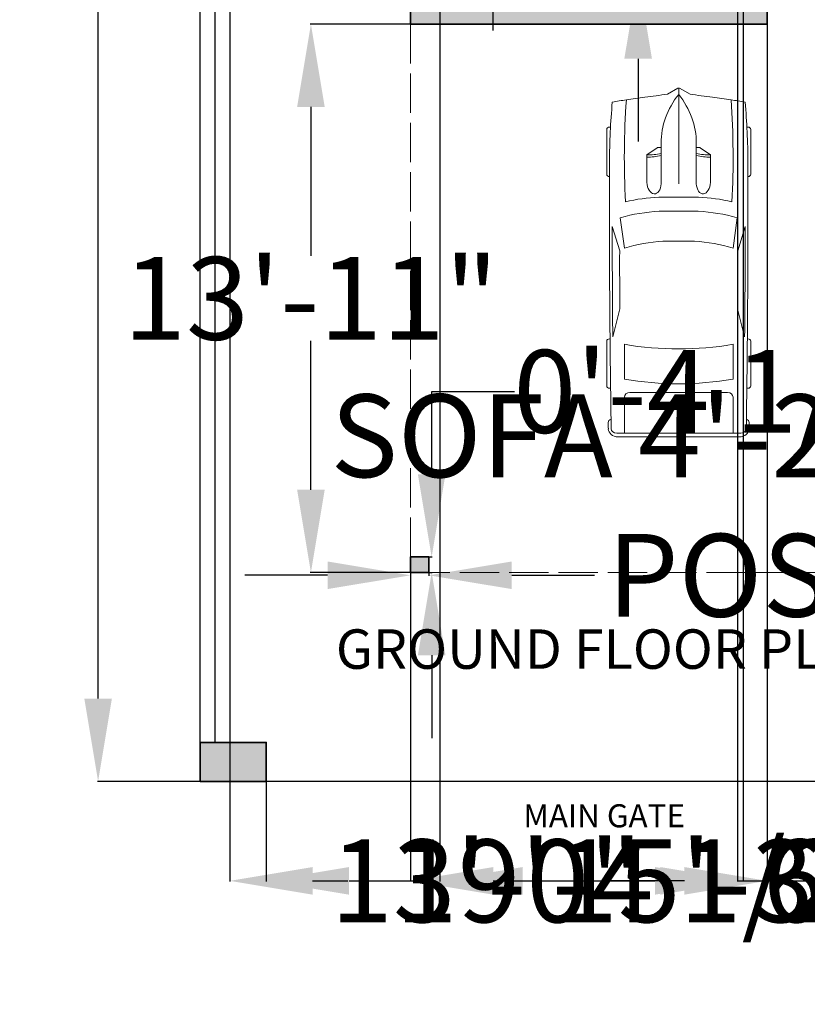
# Model space of a CAD drawing. Units: inches. Extents: x 29 to 6336, y 3 to 2592.
# Tile 1 of 8: x 5292 to 5531, y 1885 to 2184. Entities that reach past the tile are written whole.
import ezdxf

# ---------------------------------------------------------------- set-up
doc = ezdxf.new("R2010")
doc.units = ezdxf.units.IN
doc.header["$MEASUREMENT"] = 0
doc.linetypes.add('ACAD_ISO02W100', pattern=[15, 12, -3])
for name, color, linetype, lineweight in [('A-ANNO-DIMS', 2, 'Continuous', 18), ('A-ANNO-TEXT', 7, 'Continuous', 25), ('A-COLS', 7, 'Continuous', 35), ('A-COLS-PATT', 18, 'Continuous', 13), ('A-EQPM-VEHI', 8, 'Continuous', 18), ('A-FLOR-OVHD', 8, 'ACAD_ISO02W100', 18), ('A-WALL', 7, 'Continuous', 35), ('A-WALL-PATT', 242, 'Continuous', 13), ('C-PROP', 7, 'Continuous', 25)]:
    doc.layers.add(name, color=color, linetype=linetype, lineweight=lineweight)
doc.styles.get("Standard").update_dxf_attribs({"font": 'arial.ttf'})
doc.dimstyles.get("Standard").update_dxf_attribs({"dimtxt": 25.18, "dimasz": 25.18, "dimexe": 0.18, "dimexo": 0.0625, "dimgap": 0.09, "dimtad": 0, "dimtih": 1, "dimtoh": 1, "dimdec": 0, "dimzin": 0, "dimdsep": 46, "dimlunit": 3, "dimtxsty": 'Standard', "dimcen": 0.09, "dimadec": 0, "dimazin": 0, "dimtfac": 1, "dimtdec": 0, "dimtofl": 0, "dimtmove": 0, "dimatfit": 3, "dimfxl": 1, "dimtolj": 1, "dimtzin": 0, "dimarcsym": 0})

# ---------------------------------------------------------------- blocks, each defined once
blk = doc.blocks.new('*D6')
at = {"layer": 'A-ANNO-DIMS', "color": 0, "lineweight": -2, "transparency": 16777216}
for p, q in [((5346.6, 2492.39), (5315.46, 2492.39)), ((5315.64, 2467.21), (5315.64, 2235.26)), ((5315.64, 1977.51), (5315.64, 2209.47)), ((5346.6, 1952.33), (5315.46, 1952.33))]:
    blk.add_line(p, q, dxfattribs=at)
at = {"layer": 'A-ANNO-DIMS', "color": 0, "transparency": 16777216}
for points in [[(5311.44, 2467.21), (5319.83, 2467.21), (5315.64, 2492.39)], [(5311.44, 1977.51), (5319.83, 1977.51), (5315.64, 1952.33)]]:
    blk.add_solid(points, dxfattribs=at)
at = {"layer": 'Defpoints', "color": 0, "transparency": 16777216}
for p in [(5346.66, 2492.39), (5315.64, 1952.33), (5346.66, 1952.33)]:
    blk.add_point(p, dxfattribs=at)
at = {"layer": 'A-ANNO-DIMS', "color": 0, "transparency": 16777216, "insert": (5315.64, 2222.36), "char_height": 25.18, "attachment_point": 5}
blk.add_mtext("\\A1;45'", dxfattribs=at)
blk = doc.blocks.new('*U8')
for p, q in [((21.1, 37.41), (21.1, 36.83)), ((46.55, 38.89), (22.35, 38.89)), ((47.8, 37.39), (47.8, 37.41)), ((135.45, 37.07), (135.45, 37.41)), ((136.7, 38.89), (160.9, 38.89)), ((162.15, 37.41), (162.15, 36.77)), ((87.99, 31.87), (74.76, 35.92)), ((134.31, 35.6), (119.29, 31.78)), ((186.47, -33.5), (186.47, 33.5)), ((188.4, -32.76), (188.4, 32.76)), ((70.03, 31.54), (86.41, 29.35)), ((138.42, 29.35), (157.25, 29.35)), ((186.47, 29.35), (167.01, 29.35)), ((164.52, 26.39), (164.52, -26.39)), ((32.27, 11.63), (36.13, 17.17)), ((36.13, 17.17), (50.94, 17.17)), ((32.12, 9.51), (32.12, 11.15)), ((58.92, -10.77), (58.92, 10.77)), ((3.27, 6.13), (0.1, 0.41)), ((29.77, 9.51), (51.68, 9.51)), ((66.55, -10.53), (66.55, 10.53)), ((82.74, 8.5), (82.74, -8.5)), ((186.47, -10.53), (186.47, 10.53)), ((0, 0), (51.68, 0)), ((0.1, -0.41), (3.27, -6.13)), ((29.77, -9.51), (51.68, -9.51)), ((32.12, -9.51), (32.12, -11.15)), ((32.27, -11.63), (36.13, -17.17)), ((36.13, -17.17), (50.94, -17.17)), ((86.41, -29.35), (70.03, -31.54)), ((87.99, -31.87), (74.76, -35.92)), ((134.31, -35.6), (119.29, -31.78)), ((157.25, -29.35), (138.42, -29.35)), ((167.01, -29.35), (186.47, -29.35)), ((21.1, -37.41), (21.1, -36.83)), ((135.45, -37.07), (135.45, -37.41)), ((162.15, -37.41), (162.15, -36.77)), ((46.55, -38.89), (22.35, -38.89)), ((47.8, -37.39), (47.8, -37.41)), ((136.7, -38.89), (160.9, -38.89))]:
    blk.add_line(p, q)
for centre, major_axis, ratio, start_param, end_param in [((41.19, -490.86), (0, 528.23), 0.842304, 0.00281, 0.075598), ((22.35, 37.41), (0, -1.48), 0.842304, 3.141593, 4.712389), ((64.48, -10555.62), (0, 10593.03), 0.842304, -0.013397, 0.002797), ((46.55, 37.41), (0, 1.48), 0.842304, -1.570796, 0), ((136.7, 37.41), (0, -1.48), 0.842304, 3.141593, 4.712389), ((160.9, 37.41), (0, 1.48), 0.842304, -1.570796, 0), ((180.63, 35.84), (0, 2.22), 0.842304, -0.013017, 1.249894), ((64.48, -10556.36), (0, 10595.31), 0.842304, -0.013397, -0.013017), ((183.98, 32.76), (0, -5.25), 0.842304, 1.570796, 3.128196), ((266.03, -27.52), (0, 313.31), 0.842304, 1.367076, 1.39176), ((64.48, -10555.62), (0, -10591.55), 0.842304, 3.133765, 3.140441), ((183.98, 33.5), (0, -2.96), 0.842304, 1.570796, 3.128196), ((259.18, -27.52), (0, -305.3), 0.842304, 4.528606, 4.561838), ((37.47, -593.96), (0, -623.33), 0.842304, 3.096046, 3.200911), ((134.4, 5.39), (0, -89.78), 0.842304, 4.449482, 4.652344), ((135.29, 5.39), (0, 81.77), 0.842304, 1.245306, 1.50788), ((149.6, 2.8), (0, -79.58), 0.842304, 4.372215, 4.640744), ((95.79, -3666.35), (0, -3698.24), 0.842304, 3.134049, 3.144098), ((17.08, 0), (0, 147.02), 0.842304, 4.511394, 4.913384), ((35.91, 0), (0, 147.02), 0.842304, 4.511394, 4.913384), ((167.01, 26.39), (0, 2.96), 0.842304, 0, 1.570796), ((-204.49, 52.4), (0, -250.96), 0.842304, 1.385369, 1.434372), ((13.04, 17.01), (0, 27.42), 0.842304, 4.435146, 4.718221), ((14.2, 17.01), (0, 27.42), 0.842304, 4.435146, 4.718221), ((50.79, 13.34), (6.34, -0.36), 0.603834, -1.395552, 1.581315), ((32.75, 11.15), (0, 0.74), 0.842304, 0.879714, 1.570796), ((29.77, -46.66), (0, 56.17), 0.842304, 0, 0.590319), ((0.62, 0), (0, -0.74), 0.842304, 4.131459, 5.293319), ((29.77, 46.66), (0, 56.17), 0.842304, 2.551274, 3.141593), ((-204.49, -52.4), (0, 250.96), 0.842304, -1.434372, -1.385369), ((13.04, -17.01), (0, -27.42), 0.842304, 1.564964, 1.848039), ((14.2, -17.01), (0, -27.42), 0.842304, 1.564964, 1.848039), ((135.29, -5.39), (0, -81.77), 0.842304, -1.50788, -1.245306), ((149.6, -2.8), (0, -79.58), 0.842304, -1.499151, -1.230623), ((32.75, -11.15), (0, -0.74), 0.842304, 4.712389, 5.403472), ((134.4, -5.39), (0, -89.78), 0.842304, -1.510751, -1.307889), ((259.18, 27.52), (0, 305.3), 0.842304, 1.721348, 1.754579), ((167.01, -26.39), (0, -2.96), 0.842304, 4.712389, 6.283185), ((266.03, 27.52), (0, 313.31), 0.842304, 1.749832, 1.774517), ((37.47, 593.96), (0, -623.33), 0.842304, -0.059319, 0.045547), ((95.79, 3666.35), (0, -3698.24), 0.842304, -0.002505, 0.007544), ((41.19, 490.86), (0, -528.23), 0.842304, -0.075598, -0.00281), ((64.48, 10555.62), (0, 10593.03), 0.842304, 3.138796, 3.15499), ((64.48, 10555.62), (0, -10591.55), 0.842304, 0.001152, 0.007828), ((180.63, -35.84), (0, -2.22), 0.842304, -1.249894, 0.013017), ((183.98, -33.5), (0, 2.96), 0.842304, 3.15499, 4.712389), ((183.98, -32.76), (0, -5.25), 0.842304, 0.013397, 1.570796), ((22.35, -37.41), (0, 1.48), 0.842304, 1.570796, 3.141593), ((46.55, -37.41), (0, -1.48), 0.842304, 0, 1.570796), ((136.7, -37.41), (0, -1.48), 0.842304, -1.570796, 0), ((160.9, -37.41), (0, 1.48), 0.842304, 3.141593, 4.712389), ((64.48, 10556.36), (0, 10595.31), 0.842304, 3.15461, 3.15499)]:
    blk.add_ellipse(centre, major_axis=major_axis, ratio=ratio, start_param=start_param, end_param=end_param)
at = {"extrusion": (0, 0, -1)}
blk.add_ellipse((50.79, -13.34), major_axis=(6.34, 0.36), ratio=0.603834, start_param=-1.395552, end_param=1.581315, dxfattribs=at)
blk = doc.blocks.new('PORCH-POST')
blk.add_lwpolyline([(5.63, 0), (0, 0), (0, 4.72), (5.63, 4.72)], close=True)
blk = doc.blocks.new('*D25')
at = {"layer": 'A-ANNO-DIMS', "color": 0, "lineweight": -2, "transparency": 16777216}
for p, q in [((5435.68, 2266.92), (5435.68, 2292.1)), ((5435.68, 2292.1), (5460.86, 2292.1)), ((5437.84, 2241.74), (5435.5, 2241.74)), ((5437.84, 2231.12), (5435.5, 2231.12)), ((5435.68, 2205.94), (5435.68, 2180.76))]:
    blk.add_line(p, q, dxfattribs=at)
at = {"layer": 'A-ANNO-DIMS', "color": 0, "transparency": 16777216}
for points in [[(5431.49, 2266.92), (5439.88, 2266.92), (5435.68, 2241.74)], [(5431.49, 2205.94), (5439.88, 2205.94), (5435.68, 2231.12)]]:
    blk.add_solid(points, dxfattribs=at)
at = {"layer": 'Defpoints', "color": 0, "transparency": 16777216}
for p in [(5435.68, 2241.74), (5437.91, 2241.74), (5437.91, 2231.12)]:
    blk.add_point(p, dxfattribs=at)
at = {"layer": 'A-ANNO-DIMS', "color": 0, "transparency": 16777216, "insert": (5576.81, 2292.1), "char_height": 25.18, "attachment_point": 5}
blk.add_mtext('\\A1;0\'-10 1/2" TYP.', dxfattribs=at)
blk = doc.blocks.new('*D28')
at = {"layer": 'A-ANNO-DIMS', "color": 0, "lineweight": -2, "transparency": 16777216}
for p, q in [((5689.81, 2064.89), (5689.81, 2057.28)), ((5739.75, 2064.89), (5739.75, 2057.28)), ((5664.63, 2057.46), (5639.45, 2057.46)), ((5764.93, 2057.46), (5790.11, 2057.46))]:
    blk.add_line(p, q, dxfattribs=at)
at = {"layer": 'A-ANNO-DIMS', "color": 0, "transparency": 16777216}
for points in [[(5664.63, 2061.65), (5664.63, 2053.26), (5689.81, 2057.46)], [(5764.93, 2061.65), (5764.93, 2053.26), (5739.75, 2057.46)]]:
    blk.add_solid(points, dxfattribs=at)
at = {"layer": 'Defpoints', "color": 0, "transparency": 16777216}
for p in [(5689.81, 2064.95), (5739.75, 2064.95), (5689.81, 2057.46)]:
    blk.add_point(p, dxfattribs=at)
at = {"layer": 'A-ANNO-DIMS', "color": 0, "transparency": 16777216, "insert": (5509.91, 2057.46), "char_height": 25.18, "attachment_point": 5}
blk.add_mtext('\\A1;SOFA 4\'-2" TYP.', dxfattribs=at)
blk = doc.blocks.new('*D38')
at = {"layer": 'A-ANNO-DIMS', "color": 0, "lineweight": -2, "transparency": 16777216}
for p, q in [((5410.6, 2015.81), (5410.6, 2014.84)), ((5416.23, 2015.81), (5416.23, 2014.84)), ((5385.42, 2015.02), (5360.24, 2015.02)), ((5441.41, 2015.02), (5466.59, 2015.02))]:
    blk.add_line(p, q, dxfattribs=at)
at = {"layer": 'A-ANNO-DIMS', "color": 0, "transparency": 16777216}
for points in [[(5385.42, 2019.22), (5385.42, 2010.83), (5410.6, 2015.02)], [(5441.41, 2019.22), (5441.41, 2010.83), (5416.23, 2015.02)]]:
    blk.add_solid(points, dxfattribs=at)
at = {"layer": 'Defpoints', "color": 0, "transparency": 16777216}
for p in [(5410.6, 2015.87), (5416.23, 2015.87), (5416.23, 2015.02)]:
    blk.add_point(p, dxfattribs=at)
at = {"layer": 'A-ANNO-DIMS', "color": 0, "transparency": 16777216, "insert": (5624.9, 2015.02), "char_height": 25.18, "attachment_point": 5}
blk.add_mtext('\\A1;POST 0\'-5 1/2" TYP.', dxfattribs=at)
blk = doc.blocks.new('*D39')
at = {"layer": 'A-ANNO-DIMS', "color": 0, "lineweight": -2, "transparency": 16777216}
for p, q in [((5417.07, 2045.77), (5417.07, 2070.95)), ((5417.07, 2070.95), (5442.25, 2070.95)), ((5416.29, 2020.59), (5417.25, 2020.59)), ((5416.29, 2015.87), (5417.25, 2015.87)), ((5417.07, 1990.69), (5417.07, 1965.51))]:
    blk.add_line(p, q, dxfattribs=at)
at = {"layer": 'A-ANNO-DIMS', "color": 0, "transparency": 16777216}
for points in [[(5412.88, 2045.77), (5421.27, 2045.77), (5417.07, 2020.59)], [(5412.88, 1990.69), (5421.27, 1990.69), (5417.07, 2015.87)]]:
    blk.add_solid(points, dxfattribs=at)
at = {"layer": 'Defpoints', "color": 0, "transparency": 16777216}
for p in [(5416.23, 2020.59), (5417.07, 2020.59), (5416.23, 2015.87)]:
    blk.add_point(p, dxfattribs=at)
at = {"layer": 'A-ANNO-DIMS', "color": 0, "transparency": 16777216, "insert": (5548.42, 2070.95), "char_height": 25.18, "attachment_point": 5}
blk.add_mtext('\\A1;0\'-4 1/2" TYP.', dxfattribs=at)
blk = doc.blocks.new('*D42')
at = {"layer": 'A-ANNO-DIMS', "color": 0, "lineweight": -2, "transparency": 16777216}
for p, q in [((5511.77, 2337.07), (5511.77, 1921.9)), ((5355.66, 2328.5), (5355.66, 1921.9)), ((5380.84, 1922.08), (5391.56, 1922.08)), ((5486.59, 1922.08), (5475.87, 1922.08))]:
    blk.add_line(p, q, dxfattribs=at)
at = {"layer": 'A-ANNO-DIMS', "color": 0, "transparency": 16777216}
for points in [[(5380.84, 1926.28), (5380.84, 1917.88), (5355.66, 1922.08)], [(5486.59, 1926.28), (5486.59, 1917.88), (5511.77, 1922.08)]]:
    blk.add_solid(points, dxfattribs=at)
at = {"layer": 'Defpoints', "color": 0, "transparency": 16777216}
for p in [(5511.77, 2337.13), (5355.66, 2328.56), (5511.77, 1922.08)]:
    blk.add_point(p, dxfattribs=at)
at = {"layer": 'A-ANNO-DIMS', "color": 0, "transparency": 16777216, "insert": (5433.71, 1922.08), "char_height": 25.18, "attachment_point": 5}
blk.add_mtext('\\A1;13\'-0"', dxfattribs=at)
blk = doc.blocks.new('*D49')
at = {"layer": 'A-ANNO-DIMS', "color": 0, "lineweight": -2, "transparency": 16777216}
for p, q in [((5419.6, 2191.59), (5419.6, 1921.9)), ((5510.11, 2191.59), (5510.11, 1921.9)), ((5444.78, 1922.08), (5484.93, 1922.08)), ((5510.11, 1922.08), (5535.29, 1922.08))]:
    blk.add_line(p, q, dxfattribs=at)
at = {"layer": 'A-ANNO-DIMS', "color": 0, "transparency": 16777216}
for points in [[(5444.78, 1926.28), (5444.78, 1917.88), (5419.6, 1922.08)], [(5484.93, 1926.28), (5484.93, 1917.88), (5510.11, 1922.08)]]:
    blk.add_solid(points, dxfattribs=at)
at = {"layer": 'Defpoints', "color": 0, "transparency": 16777216}
for p in [(5419.6, 2191.65), (5510.11, 2191.65), (5510.11, 1922.08)]:
    blk.add_point(p, dxfattribs=at)
at = {"layer": 'A-ANNO-DIMS', "color": 0, "transparency": 16777216, "insert": (5598.08, 1922.08), "char_height": 25.18, "attachment_point": 5}
blk.add_mtext('\\A1;7\'-6 1/2"', dxfattribs=at)
blk = doc.blocks.new('*D56')
at = {"layer": 'A-ANNO-DIMS', "color": 0, "lineweight": -2, "transparency": 16777216}
for p, q in [((5366.79, 1952.27), (5366.79, 1921.9)), ((5599.23, 1952.27), (5599.23, 1921.9)), ((5391.97, 1922.08), (5411.52, 1922.08)), ((5574.05, 1922.08), (5554.5, 1922.08))]:
    blk.add_line(p, q, dxfattribs=at)
at = {"layer": 'A-ANNO-DIMS', "color": 0, "transparency": 16777216}
for points in [[(5391.97, 1926.28), (5391.97, 1917.88), (5366.79, 1922.08)], [(5574.05, 1926.28), (5574.05, 1917.88), (5599.23, 1922.08)]]:
    blk.add_solid(points, dxfattribs=at)
at = {"layer": 'Defpoints', "color": 0, "transparency": 16777216}
for p in [(5366.79, 1952.33), (5599.23, 1952.33), (5599.23, 1922.08)]:
    blk.add_point(p, dxfattribs=at)
at = {"layer": 'A-ANNO-DIMS', "color": 0, "transparency": 16777216, "insert": (5483.01, 1922.08), "char_height": 25.18, "attachment_point": 5}
blk.add_mtext('\\A1;19\'-4 1/2"', dxfattribs=at)
blk = doc.blocks.new('*D57')
at = {"layer": 'A-ANNO-DIMS', "color": 0, "lineweight": -2, "transparency": 16777216}
for p, q in [((5410.6, 2015.81), (5410.6, 1921.9)), ((5593.6, 2015.81), (5593.6, 1921.9)), ((5435.78, 1922.08), (5459.94, 1922.08)), ((5568.42, 1922.08), (5544.25, 1922.08))]:
    blk.add_line(p, q, dxfattribs=at)
at = {"layer": 'A-ANNO-DIMS', "color": 0, "transparency": 16777216}
for points in [[(5435.78, 1926.28), (5435.78, 1917.88), (5410.6, 1922.08)], [(5568.42, 1926.28), (5568.42, 1917.88), (5593.6, 1922.08)]]:
    blk.add_solid(points, dxfattribs=at)
at = {"layer": 'Defpoints', "color": 0, "transparency": 16777216}
for p in [(5410.6, 2015.87), (5593.6, 2015.87), (5593.6, 1922.08)]:
    blk.add_point(p, dxfattribs=at)
at = {"layer": 'A-ANNO-DIMS', "color": 0, "transparency": 16777216, "insert": (5502.1, 1922.08), "char_height": 25.18, "attachment_point": 5}
blk.add_mtext('\\A1;15\'-3"', dxfattribs=at)
blk = doc.blocks.new('*D58')
at = {"layer": 'A-ANNO-DIMS', "color": 0, "lineweight": -2, "transparency": 16777216}
for p, q in [((5410.54, 2182.65), (5380.17, 2182.65)), ((5380.35, 2157.47), (5380.35, 2112.21)), ((5380.35, 2041.05), (5380.35, 2086.3)), ((5410.54, 2015.87), (5380.17, 2015.87))]:
    blk.add_line(p, q, dxfattribs=at)
at = {"layer": 'A-ANNO-DIMS', "color": 0, "transparency": 16777216}
for points in [[(5376.16, 2157.47), (5384.55, 2157.47), (5380.35, 2182.65)], [(5376.16, 2041.05), (5384.55, 2041.05), (5380.35, 2015.87)]]:
    blk.add_solid(points, dxfattribs=at)
at = {"layer": 'Defpoints', "color": 0, "transparency": 16777216}
for p in [(5380.35, 2182.65), (5410.6, 2182.65), (5410.6, 2015.87)]:
    blk.add_point(p, dxfattribs=at)
at = {"layer": 'A-ANNO-DIMS', "color": 0, "transparency": 16777216, "insert": (5380.35, 2099.26), "char_height": 25.18, "attachment_point": 5}
blk.add_mtext('\\A1;13\'-11"', dxfattribs=at)
blk = doc.blocks.new('*D59')
at = {"layer": 'A-ANNO-DIMS', "color": 0, "lineweight": -2, "transparency": 16777216}
for p, q in [((5519.11, 2182.59), (5519.11, 1921.9)), ((5592.36, 2182.59), (5592.36, 1921.9)), ((5493.93, 1922.08), (5468.75, 1922.08)), ((5617.54, 1922.08), (5642.72, 1922.08))]:
    blk.add_line(p, q, dxfattribs=at)
at = {"layer": 'A-ANNO-DIMS', "color": 0, "transparency": 16777216}
for points in [[(5493.93, 1926.28), (5493.93, 1917.88), (5519.11, 1922.08)], [(5617.54, 1926.28), (5617.54, 1917.88), (5592.36, 1922.08)]]:
    blk.add_solid(points, dxfattribs=at)
at = {"layer": 'Defpoints', "color": 0, "transparency": 16777216}
for p in [(5519.11, 2182.65), (5592.36, 2182.65), (5592.36, 1922.08)]:
    blk.add_point(p, dxfattribs=at)
at = {"layer": 'A-ANNO-DIMS', "color": 0, "transparency": 16777216, "insert": (5555.73, 1922.08), "char_height": 25.18, "attachment_point": 5}
blk.add_mtext('\\A1;6\'-1"', dxfattribs=at)
blk = doc.blocks.new('*D68')
at = {"layer": 'A-ANNO-DIMS', "color": 0, "lineweight": -2, "transparency": 16777216}
for p, q in [((5479.86, 2259.85), (5479.86, 2285.03)), ((5510.05, 2234.67), (5479.68, 2234.67)), ((5510.05, 2197.33), (5479.68, 2197.33)), ((5479.86, 2172.15), (5479.86, 2146.97))]:
    blk.add_line(p, q, dxfattribs=at)
at = {"layer": 'A-ANNO-DIMS', "color": 0, "transparency": 16777216}
for points in [[(5475.66, 2259.85), (5484.06, 2259.85), (5479.86, 2234.67)], [(5475.66, 2172.15), (5484.06, 2172.15), (5479.86, 2197.33)]]:
    blk.add_solid(points, dxfattribs=at)
at = {"layer": 'Defpoints', "color": 0, "transparency": 16777216}
for p in [(5479.86, 2234.67), (5510.11, 2234.67), (5510.11, 2197.33)]:
    blk.add_point(p, dxfattribs=at)
at = {"layer": 'A-ANNO-DIMS', "color": 0, "transparency": 16777216, "insert": (5479.86, 2216), "char_height": 25.18, "attachment_point": 5}
blk.add_mtext('\\A1;3\'-1 1/2"', dxfattribs=at)

msp = doc.modelspace()

# ---------------------------------------------------------------- hatches: boundary and pattern name
at = {"layer": 'A-COLS-PATT'}
h = msp.add_hatch(color=256, dxfattribs=at)
h.dxf.hatch_style = 1
h.paths.add_polyline_path([(5416.23, 2020.59), (5410.6, 2020.59), (5410.6, 2015.87), (5416.23, 2015.87)])
h.paths.add_polyline_path([(5599.23, 2020.59), (5593.6, 2020.59), (5593.6, 2015.87), (5599.23, 2015.87)])
h = msp.add_hatch(color=256, dxfattribs=at)
h.dxf.hatch_style = 1
h.paths.add_polyline_path([(5366.79, 1964.19), (5346.66, 1964.19), (5346.66, 1952.33), (5366.79, 1952.33)])
at = {"layer": 'A-WALL-PATT'}
h = msp.add_hatch(color=256, dxfattribs=at)
h.dxf.hatch_style = 1
h.paths.add_polyline_path([(5558.68, 2492.33), (5459.71, 2492.33), (5459.71, 2483.33), (5511.77, 2483.33), (5511.77, 2388.68), (5520.77, 2388.68), (5520.77, 2393.05), (5526.31, 2393.05), (5526.31, 2402.05), (5520.77, 2402.05), (5520.77, 2483.33), (5558.68, 2483.33)])
h.paths.add_polyline_path([(5659.13, 2492.33), (5586.68, 2492.33), (5586.68, 2483.33), (5624.6, 2483.33), (5624.6, 2402.05), (5562.29, 2402.05), (5562.29, 2393.05), (5676.48, 2393.05), (5676.48, 2402.05), (5633.6, 2402.05), (5633.6, 2422.71), (5633.6, 2483.33), (5659.13, 2483.33)])
h.paths.add_polyline_path([(5886.66, 2492.33), (5687.13, 2492.33), (5687.13, 2483.33), (5712.66, 2483.33), (5712.66, 2468.69), (5721.66, 2468.69), (5721.66, 2483.33), (5877.66, 2483.33), (5877.66, 2106.48), (5858.21, 2106.48), (5858.21, 2097.48), (5877.66, 2097.48), (5877.66, 1961.33), (5877.66, 1952.33), (5886.66, 1952.33)])
h.paths.add_polyline_path([(5721.66, 2416.69), (5712.66, 2416.69), (5712.66, 2402.05), (5709.45, 2402.05), (5709.45, 2393.05), (5712.66, 2393.05), (5712.66, 2386.01), (5721.66, 2386.01)], flags=17)
h.paths.add_polyline_path([(5355.66, 2483.33), (5407.71, 2483.33), (5407.71, 2492.33), (5346.66, 2492.33), (5346.66, 2431.95), (5355.66, 2431.95)])
h.paths.add_polyline_path([(5355.66, 2379.95), (5346.66, 2379.95), (5346.66, 2319.56), (5355.66, 2319.56), (5355.66, 2328.56)])
h.paths.add_polyline_path([(5520.77, 2337.13), (5511.77, 2337.13), (5511.77, 2328.56), (5410.6, 2328.56), (5410.6, 2319.56), (5410.6, 2281.61), (5419.6, 2281.61), (5419.6, 2319.56), (5510.11, 2319.56), (5510.11, 2234.67), (5519.11, 2234.67), (5519.11, 2319.56), (5520.77, 2319.56)])
h.paths.add_polyline_path([(5519.11, 2197.33), (5510.11, 2197.33), (5510.11, 2191.65), (5419.6, 2191.65), (5419.6, 2228.6), (5419.6, 2229.61), (5410.6, 2229.61), (5410.6, 2182.65), (5519.11, 2182.65)])
h.paths.add_polyline_path([(5712.66, 2193.6), (5592.36, 2193.6), (5592.36, 2182.65), (5624.77, 2182.65), (5633.77, 2182.65), (5712.66, 2182.65)])
h.paths.add_polyline_path([(5633.77, 2182.65), (5624.77, 2182.65), (5624.77, 2051.72), (5633.77, 2051.72), (5691.77, 2051.72), (5691.77, 2060.72), (5633.77, 2060.72)])
h.paths.add_polyline_path([(5810.76, 2097.48), (5830.21, 2097.48), (5830.21, 2106.48), (5810.76, 2106.48), (5810.76, 2182.65), (5817.87, 2182.65), (5817.87, 2193.6), (5783.59, 2193.6), (5783.59, 2182.65), (5801.76, 2182.65), (5801.76, 2060.72), (5743.77, 2060.72), (5743.77, 2051.72), (5810.76, 2051.72)], flags=17)
h.paths.add_polyline_path([(5721.66, 2319.56), (5877.66, 2319.56), (5877.66, 2328.56), (5721.66, 2328.56), (5721.66, 2335.85), (5712.66, 2335.85), (5712.66, 2319.56), (5712.66, 2182.65), (5726.12, 2182.65), (5726.12, 2193.6), (5721.66, 2193.6)], flags=17)
h.paths.add_polyline_path([(5631.73, 2431.78), (5711.31, 2431.78), (5711.31, 2446.2), (5631.73, 2446.2)], flags=9)

# ---------------------------------------------------------------- linework, layer by layer
at = {"layer": 'A-COLS'}
msp.add_lwpolyline([(5346.66, 1964.19), (5366.79, 1964.19), (5366.79, 1952.33), (5346.66, 1952.33)], close=True, dxfattribs=at)
at = {"layer": 'A-FLOR-OVHD'}
for p, q in [((5410.6, 2182.65), (5410.6, 2015.87)), ((5410.6, 2015.87), (5599.23, 2015.87))]:
    msp.add_line(p, q, dxfattribs=at)
at = {"layer": 'A-WALL'}
for p, q in [((5410.6, 2182.65), (5410.6, 2319.56)), ((5519.11, 2182.65), (5519.11, 2197.33)), ((5410.6, 2182.65), (5519.11, 2182.65))]:
    msp.add_line(p, q, dxfattribs=at)
at = {"layer": 'C-PROP'}
for p, q in [((5346.66, 1952.33), (5346.66, 2492.33)), ((5351.16, 2319.56), (5351.16, 1964.19)), ((5886.66, 1952.33), (5346.66, 1952.33))]:
    msp.add_line(p, q, dxfattribs=at)

# ---------------------------------------------------------------- block references
at = {"layer": 'A-COLS'}
msp.add_blockref('PORCH-POST', (5410.6, 2015.87), dxfattribs=at)
at = {"layer": 'A-EQPM-VEHI', "xscale": 0.5630739154895661, "yscale": 0.5630739154895661, "zscale": 0.5630739154895661, "rotation": 270}
msp.add_blockref('*U8', (5492.19, 2163.22), dxfattribs=at)

# ---------------------------------------------------------------- texts
at = {"layer": 'A-ANNO-TEXT', "attachment_point": 1}
for s, width, insert, char_height in [('GROUND FLOOR PLAN', 221.0762, (5387.94, 1998.58), 12), ('MAIN GATE', 54.3344, (5444.95, 1945.37), 7)]:
    msp.add_mtext_dynamic_manual_height_columns(s, width=width, gutter_width=1, heights=[0], dxfattribs=dict(at, insert=insert, char_height=char_height))

# ---------------------------------------------------------------- dimensions: what is measured, and where the dimension line sits
at = {"layer": 'A-ANNO-DIMS'}
for base, p1, p2, override, picture, middle in [((5315.64, 1952.33), (5346.66, 2492.39), (5346.66, 1952.33), {"dimclrd": 0, "dimclre": 0, "dimclrt": 0}, '*D6', (5315.64, 2222.36)), ((5479.86, 2234.67), (5510.11, 2197.33), (5510.11, 2234.67), {"dimdec": 1, "dimlfac": 1, "dimrnd": 0, "dimzin": 1, "dimdsep": 46, "dimlunit": 4, "dimfrac": 2}, '*D68', (5479.86, 2216)), ((5380.35, 2182.65), (5410.6, 2015.87), (5410.6, 2182.65), {"dimdec": 1, "dimlfac": 1, "dimrnd": 0, "dimzin": 1, "dimdsep": 46, "dimlunit": 4, "dimfrac": 2}, '*D58', (5380.35, 2099.26))]:
    dim = msp.add_linear_dim(base=base, p1=p1, p2=p2, angle=90, dimstyle='Standard', override=override, dxfattribs=at)
    dim.commit()
    dim.dimension.update_dxf_attribs({"geometry": picture, "text_midpoint": middle})
for base, p1, p2, angle, text, picture, middle in [((5435.68, 2241.74), (5437.91, 2231.12), (5437.91, 2241.74), 90, '<> TYP.', '*D25', (5576.81, 2292.1)), ((5417.07, 2020.59), (5416.23, 2015.87), (5416.23, 2020.59), 90, '<> TYP.', '*D39', (5548.42, 2070.95)), ((5689.81, 2057.46), (5739.75, 2064.95), (5689.81, 2064.95), 180, 'SOFA <> TYP.', '*D28', (5509.91, 2057.46))]:
    dim = msp.add_linear_dim(base=base, p1=p1, p2=p2, angle=angle, text=text, dimstyle='Standard', override={"dimdec": 1, "dimlfac": 1, "dimrnd": 0, "dimzin": 1, "dimdsep": 46, "dimlunit": 4, "dimfrac": 2}, dxfattribs=at)
    dim.commit()
    dim.dimension.update_dxf_attribs({"geometry": picture, "text_midpoint": middle})
for base, p1, p2, picture, middle in [((5511.77, 1922.08), (5355.66, 2328.56), (5511.77, 2337.13), '*D42', (5433.71, 1922.08)), ((5510.11, 1922.08), (5419.6, 2191.65), (5510.11, 2191.65), '*D49', (5598.08, 1922.08)), ((5592.3592, 1922.0797), (5519.1102, 2182.6481), (5592.3592, 2182.6517), '*D59', (5555.7347, 1922.0797)), ((5593.6, 1922.08), (5410.6, 2015.87), (5593.6, 2015.87), '*D57', (5502.1, 1922.08)), ((5599.23, 1922.08), (5366.79, 1952.33), (5599.23, 1952.33), '*D56', (5483.01, 1922.08))]:
    dim = msp.add_linear_dim(base=base, p1=p1, p2=p2, dimstyle='Standard', override={"dimdec": 1, "dimlfac": 1, "dimrnd": 0, "dimzin": 1, "dimdsep": 46, "dimlunit": 4, "dimfrac": 2}, dxfattribs=at)
    dim.commit()
    dim.dimension.update_dxf_attribs({"geometry": picture, "text_midpoint": middle})
dim = msp.add_linear_dim(base=(5416.23, 2015.02), p1=(5410.6, 2015.87), p2=(5416.23, 2015.87), text='POST <> TYP.', dimstyle='Standard', override={"dimdec": 1, "dimlfac": 1, "dimrnd": 0, "dimzin": 1, "dimdsep": 46, "dimlunit": 4, "dimfrac": 2}, dxfattribs=at)
dim.commit()
dim.dimension.update_dxf_attribs({"geometry": '*D38', "text_midpoint": (5624.9, 2015.02)})

doc.saveas('drawing.dxf')
